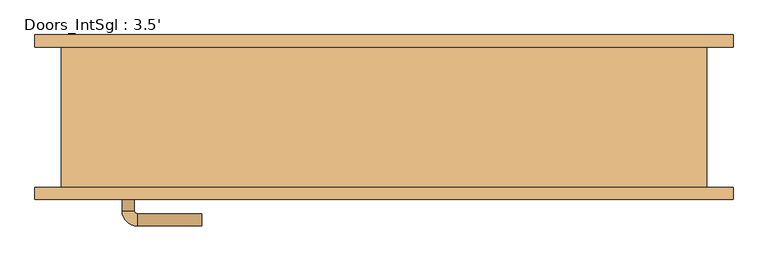
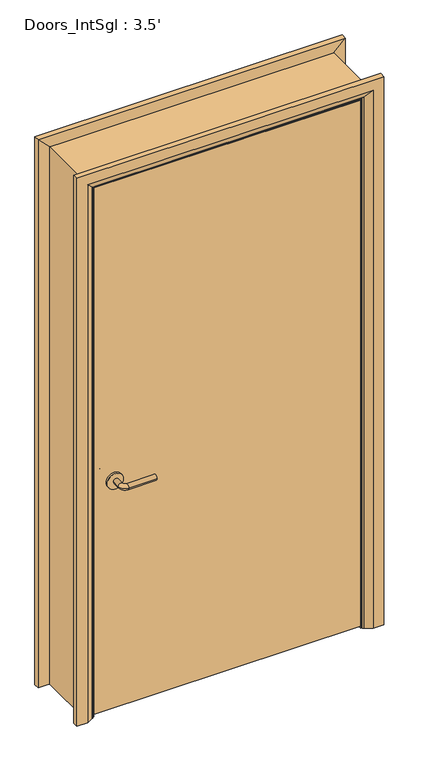
"""IFC4 building model written with IfcOpenShell, lengths in millimetres: door geometry, Doors_IntSgl : 3.5'."""

from ifc_helpers import new_model, si_unit, point, frame, frame_2d, origin, place, context, project, spatial, polyline, circle_curve, ellipse_curve, trimmed, segment, composite_curve, outline, extrude, faceted_brep, source, transform, mapped, element, save
from ifc_brep_helpers import plane_surface, cylinder_surface, revolved_surface, advanced_brep


def doors_intsgl_3_5_83ebdd9c(model_context):
    return source(origin(), model_context, "Body", "SolidModel", [
        advanced_brep(
        [(-426.4, -68.3, 900.0), (-406.4, -68.3, 900.0), (-426.4, -38.3, 900.0), (-406.4, -38.3, 900.0), (-401.4, -33.3, 900.0), (-401.4, -13.3, 900.0), (-296.4, -13.3, 900.0), (-296.4, -33.3, 900.0)],
        [
            (0, 1, circle_curve(frame((-416.4, -68.3, 900.0), z_axis=(0.0, -1.0, 0.0), x_axis=(1.0, 0.0, 0.0)), 10.0)),
            (1, 0, circle_curve(frame((-416.4, -68.3, 900.0), z_axis=(0.0, -1.0, 0.0), x_axis=(1.0, 0.0, 0.0)), 10.0)),
            (0, 2),
            (2, 3, circle_curve(frame((-416.4, -38.3, 900.0), z_axis=(0.0, -1.0, 0.0), x_axis=(1.0, 0.0, 0.0)), 10.0)),
            (3, 1),
            (3, 2, circle_curve(frame((-416.4, -38.3, 900.0), z_axis=(0.0, -1.0, 0.0), x_axis=(1.0, 0.0, 0.0)), 10.0)),
            (4, 3, circle_curve(frame((-401.4, -38.3, 900.0), z_axis=(0.0, 0.0, 1.0), x_axis=(-1.0, 0.0, 0.0)), 5.0)),
            (2, 5, circle_curve(frame((-401.4, -38.3, 900.0), z_axis=(0.0, 0.0, -1.0), x_axis=(-1.0, 0.0, 0.0)), 25.0)),
            (5, 4, circle_curve(frame((-401.4, -23.3, 900.0), z_axis=(-1.0, 0.0, 0.0), x_axis=(0.0, -1.0, 0.0)), 10.0)),
            (4, 5, circle_curve(frame((-401.4, -23.3, 900.0), z_axis=(-1.0, 0.0, 0.0), x_axis=(0.0, -1.0, 0.0)), 10.0)),
            (6, 7, circle_curve(frame((-296.4, -23.3, 900.0), z_axis=(1.0, 0.0, 0.0), x_axis=(0.0, -1.0, 0.0)), 10.0)),
            (7, 6, circle_curve(frame((-296.4, -23.3, 900.0), z_axis=(1.0, 0.0, 0.0), x_axis=(0.0, -1.0, 0.0)), 10.0)),
            (5, 6),
            (7, 4),
        ],
        [
            plane_surface(frame((-416.4, -68.3, 900.0), z_axis=(0.0, -1.0, 0.0), x_axis=(0.0, 0.0, 1.0))),
            cylinder_surface(frame((-416.4, -68.3, 900.0), z_axis=(0.0, -1.0, 0.0), x_axis=(1.0, 0.0, 0.0)), 10.0),
            revolved_surface(trimmed(ellipse_curve(frame((-416.4, -38.3, 900.0), z_axis=(0.0, -1.0, 0.0), x_axis=(1.0, 0.0, 0.0)), 10.0, 10.0), [point((-426.4, -38.3, 900.0))], [point((-406.4, -38.3, 900.0))], True, "CARTESIAN"), (-401.4, -38.3, 900.0), (0.0, 0.0, -1.0)),
            revolved_surface(trimmed(ellipse_curve(frame((-416.4, -38.3, 900.0), z_axis=(0.0, -1.0, 0.0), x_axis=(1.0, 0.0, 0.0)), 10.0, 10.0), [point((-406.4, -38.3, 900.0))], [point((-426.4, -38.3, 900.0))], True, "CARTESIAN"), (-401.4, -38.3, 900.0), (0.0, 0.0, -1.0)),
            plane_surface(frame((-296.4, -23.3, 900.0), z_axis=(1.0, 0.0, 0.0), x_axis=(0.0, 0.0, 1.0))),
            cylinder_surface(frame((-401.4, -23.3, 900.0), z_axis=(-1.0, 0.0, 0.0), x_axis=(0.0, -1.0, 0.0)), 10.0),
        ],
        [
            (0, [[1, 2]]),
            (1, [[-1, 3, 4, 5]]),
            (1, [[-2, -5, 6, -3]]),
            (2, [[7, -4, 8, 9]]),
            (3, [[-8, -6, -7, 10]]),
            (4, [[11, 12]]),
            (5, [[-9, 13, -12, 14]]),
            (5, [[-10, -14, -11, -13]]),
        ],
    ),
        extrude(outline(composite_curve([segment(trimmed(circle_curve(frame_2d((900.0, -418.9)), 30.0), [point((900.0, -448.9))], [point((900.0, -388.9))], False, "CARTESIAN"), True, "CONTINUOUS"), segment(trimmed(circle_curve(frame_2d((900.0, -418.9)), 30.0), [point((900.0, -388.9))], [point((900.0, -448.9))], False, "CARTESIAN"), True, "CONTINUOUS")], self_intersect=False)), frame((0.0, -76.3, 0.0), z_axis=(0.0, 1.0, 0.0), x_axis=(0.0, 0.0, 1.0)), (0.0, 0.0, 1.0), 8.0),
        advanced_brep(
        [(-426.4, -122.3, 900.0), (-406.4, -122.3, 900.0), (-406.4, -152.3, 900.0), (-426.4, -152.3, 900.0), (-401.4, -157.3, 900.0), (-401.4, -177.3, 900.0), (-296.4, -177.3, 900.0), (-296.4, -157.3, 900.0)],
        [
            (0, 1, circle_curve(frame((-416.4, -122.3, 900.0), z_axis=(0.0, 1.0, 0.0), x_axis=(1.0, 0.0, 0.0)), 10.0)),
            (1, 0, circle_curve(frame((-416.4, -122.3, 900.0), z_axis=(0.0, 1.0, 0.0), x_axis=(1.0, 0.0, 0.0)), 10.0)),
            (1, 2),
            (2, 3, circle_curve(frame((-416.4, -152.3, 900.0), z_axis=(0.0, 1.0, 0.0), x_axis=(1.0, 0.0, 0.0)), 10.0)),
            (3, 0),
            (3, 2, circle_curve(frame((-416.4, -152.3, 900.0), z_axis=(0.0, 1.0, 0.0), x_axis=(1.0, 0.0, 0.0)), 10.0)),
            (4, 5, circle_curve(frame((-401.4, -167.3, 900.0), z_axis=(-1.0, 0.0, 0.0), x_axis=(0.0, 1.0, 0.0)), 10.0)),
            (5, 3, circle_curve(frame((-401.4, -152.3, 900.0), z_axis=(0.0, 0.0, -1.0), x_axis=(-1.0, 0.0, 0.0)), 25.0)),
            (2, 4, circle_curve(frame((-401.4, -152.3, 900.0), z_axis=(0.0, 0.0, 1.0), x_axis=(-1.0, 0.0, 0.0)), 5.0)),
            (5, 4, circle_curve(frame((-401.4, -167.3, 900.0), z_axis=(-1.0, 0.0, 0.0), x_axis=(0.0, 1.0, 0.0)), 10.0)),
            (6, 7, circle_curve(frame((-296.4, -167.3, 900.0), z_axis=(1.0, 0.0, 0.0), x_axis=(0.0, 1.0, 0.0)), 10.0)),
            (7, 6, circle_curve(frame((-296.4, -167.3, 900.0), z_axis=(1.0, 0.0, 0.0), x_axis=(0.0, 1.0, 0.0)), 10.0)),
            (4, 7),
            (6, 5),
        ],
        [
            plane_surface(frame((-416.4, -122.3, 900.0), z_axis=(0.0, 1.0, 0.0), x_axis=(0.0, 0.0, 1.0))),
            cylinder_surface(frame((-416.4, -122.3, 900.0), z_axis=(0.0, 1.0, 0.0), x_axis=(1.0, 0.0, 0.0)), 10.0),
            revolved_surface(trimmed(ellipse_curve(frame((-416.4, -152.3, 900.0), z_axis=(0.0, -1.0, 0.0), x_axis=(1.0, 0.0, 0.0)), 10.0, 10.0), [point((-426.4, -152.3, 900.0))], [point((-406.4, -152.3, 900.0))], True, "CARTESIAN"), (-401.4, -152.3, 900.0), (0.0, 0.0, -1.0)),
            revolved_surface(trimmed(ellipse_curve(frame((-416.4, -152.3, 900.0), z_axis=(0.0, -1.0, 0.0), x_axis=(1.0, 0.0, 0.0)), 10.0, 10.0), [point((-406.4, -152.3, 900.0))], [point((-426.4, -152.3, 900.0))], True, "CARTESIAN"), (-401.4, -152.3, 900.0), (0.0, 0.0, -1.0)),
            plane_surface(frame((-296.4, -167.3, 900.0), z_axis=(1.0, 0.0, 0.0), x_axis=(0.0, 0.0, 1.0))),
            cylinder_surface(frame((-401.4, -167.3, 900.0), z_axis=(-1.0, 0.0, 0.0), x_axis=(0.0, 1.0, 0.0)), 10.0),
        ],
        [
            (0, [[1, 2]]),
            (1, [[3, 4, 5, -2]]),
            (1, [[-5, 6, -3, -1]]),
            (2, [[7, 8, -4, 9]]),
            (3, [[10, -9, -6, -8]]),
            (4, [[11, 12]]),
            (5, [[13, -11, 14, -7]]),
            (5, [[-14, -12, -13, -10]]),
        ],
    ),
        extrude(outline(composite_curve([segment(trimmed(circle_curve(frame_2d((900.0, -418.9)), 30.0), [point((900.0, -448.9))], [point((900.0, -388.9))], False, "CARTESIAN"), True, "CONTINUOUS"), segment(trimmed(circle_curve(frame_2d((900.0, -418.9)), 30.0), [point((900.0, -388.9))], [point((900.0, -448.9))], False, "CARTESIAN"), True, "CONTINUOUS")], self_intersect=False)), frame((0.0, -122.3, 0.0), z_axis=(0.0, 1.0, 0.0), x_axis=(0.0, 0.0, 1.0)), (0.0, 0.0, 1.0), 8.0),
        extrude(outline(polyline([(491.4, -76.3), (491.4, -114.3), (-491.4, -114.3), (-491.4, -76.3), (491.4, -76.3)])), frame((0.0, 0.0, 8.0), z_axis=(0.0, 0.0, 1.0), x_axis=(1.0, 0.0, 0.0)), (0.0, 0.0, 1.0), 2060.0),
        advanced_brep(
        [(568.4, -134.3, 0.0), (528.4, -134.3, 0.0), (502.4, -120.3, 0.0), (498.4, -114.3, 0.0), (568.4, -114.3, 0.0), (568.4, -114.3, 2145.0), (568.4, -134.3, 2145.0), (498.4, -114.3, 2075.0), (-498.4, -114.3, 2075.0), (-498.4, -114.3, 0.0), (-568.4, -114.3, 0.0), (-568.4, -114.3, 2145.0), (502.4, -120.3, 2079.0), (528.4, -134.3, 2105.0), (-568.4, -134.3, 2145.0), (-568.4, -134.3, 0.0), (-528.4, -134.3, 0.0), (-528.4, -134.3, 2105.0), (-502.4, -120.3, 0.0), (-502.4, -120.3, 2079.0)],
        [
            (0, 1),
            (1, 2),
            (2, 3, circle_curve(frame((506.4, -113.3, 0.0), z_axis=(0.0, 0.0, -1.0), x_axis=(1.0, 0.0, 0.0)), 8.0622577)),
            (3, 4),
            (4, 0),
            (4, 5),
            (5, 6),
            (6, 0),
            (3, 7),
            (7, 8),
            (8, 9),
            (9, 10),
            (10, 11),
            (11, 5),
            (2, 12),
            (12, 7, ellipse_curve(frame((506.4, -113.3, 2083.0), z_axis=(0.7071067811865475, 0.0, -0.7071067811865475), x_axis=(-0.7071067811865474, 0.0, -0.7071067811865476)), 11.4017543, 8.0622577)),
            (1, 13),
            (13, 12),
            (6, 14),
            (14, 15),
            (15, 16),
            (16, 17),
            (17, 13),
            (10, 15),
            (14, 11),
            (9, 18, circle_curve(frame((-506.4, -113.3, 0.0), z_axis=(0.0, 0.0, -1.0), x_axis=(-1.0, 0.0, 0.0)), 8.0622577)),
            (18, 16),
            (19, 18),
            (8, 19, ellipse_curve(frame((-506.4, -113.3, 2083.0), z_axis=(-0.7071067811865475, 0.0, -0.7071067811865475), x_axis=(-0.7071067811865474, 0.0, 0.7071067811865476)), 11.4017543, 8.0622577)),
            (19, 17),
            (12, 19),
        ],
        [
            plane_surface(frame((498.4, -114.3, 0.0), z_axis=(0.0, 0.0, -1.0), x_axis=(0.0, 1.0, 0.0))),
            plane_surface(frame((568.4, -134.3, 0.0), z_axis=(1.0, 0.0, 0.0), x_axis=(0.0, 0.0, 1.0))),
            plane_surface(frame((568.4, -114.3, 0.0), z_axis=(0.0, 1.0, 0.0), x_axis=(0.0, 0.0, 1.0))),
            cylinder_surface(frame((506.4, -113.3, 0.0), z_axis=(0.0, 0.0, -1.0), x_axis=(1.0, 0.0, 0.0)), 8.0622577),
            plane_surface(frame((502.4, -120.3, 0.0), z_axis=(-0.4740998230350126, -0.880471099922178, 0.0), x_axis=(0.0, 0.0, 1.0))),
            plane_surface(frame((528.4, -134.3, 0.0), z_axis=(0.0, -1.0, 0.0), x_axis=(0.0, 0.0, 1.0))),
            plane_surface(frame((-568.4, -134.3, 2145.0), z_axis=(-1.0, 0.0, 0.0), x_axis=(0.0, 0.0, -1.0))),
            plane_surface(frame((-498.4, -114.3, 0.0), z_axis=(0.0, 0.0, -1.0), x_axis=(0.0, 1.0, 0.0))),
            cylinder_surface(frame((-506.4, -113.3, 2075.0), z_axis=(0.0, 0.0, 1.0), x_axis=(-1.0, 0.0, 0.0)), 8.0622577),
            plane_surface(frame((-502.4, -120.3, 2079.0), z_axis=(0.47409982303501824, -0.8804710999221749, 0.0), x_axis=(0.0, 0.0, -1.0))),
            plane_surface(frame((568.4, -134.3, 2145.0), z_axis=(0.0, 0.0, 1.0), x_axis=(-1.0, 0.0, 0.0))),
            cylinder_surface(frame((498.4, -113.3, 2083.0), z_axis=(1.0, 0.0, 0.0), x_axis=(0.0, 0.0, 1.0)), 8.0622577),
            plane_surface(frame((502.4, -120.3, 2079.0), z_axis=(0.0, -0.8804710999221764, -0.4740998230350154), x_axis=(-1.0, 0.0, 0.0))),
        ],
        [
            (0, [[1, 2, 3, 4, 5]]),
            (1, [[6, 7, 8, -5]]),
            (2, [[9, 10, 11, 12, 13, 14, -6, -4]]),
            (3, [[15, 16, -9, -3]]),
            (4, [[17, 18, -15, -2]]),
            (5, [[-8, 19, 20, 21, 22, 23, -17, -1]]),
            (6, [[-13, 24, -20, 25]]),
            (7, [[-24, -12, 26, 27, -21]]),
            (8, [[28, -26, -11, 29]]),
            (9, [[-22, -27, -28, 30]]),
            (10, [[-14, -25, -19, -7]]),
            (11, [[31, -29, -10, -16]]),
            (12, [[-23, -30, -31, -18]]),
        ],
    ),
        extrude(outline(polyline([(0.0, -474.4), (2051.0, -474.4), (2051.0, 474.4), (0.0, 474.4), (0.0, 493.4), (2070.0, 493.4), (2070.0, -493.4), (0.0, -493.4), (0.0, -474.4)])), frame((0.0, -74.3, 0.0), z_axis=(0.0, 1.0, 0.0), x_axis=(0.0, 0.0, 1.0)), (0.0, 0.0, 1.0), 32.0),
        advanced_brep(
        [(-568.4, 134.3, 0.0), (-528.4, 134.3, 0.0), (-502.4, 120.3, 0.0), (-498.4, 114.3, 0.0), (-568.4, 114.3, 0.0), (-568.4, 114.3, 2145.0), (-568.4, 134.3, 2145.0), (-498.4, 114.3, 2075.0), (-502.4, 120.3, 2079.0), (-528.4, 134.3, 2105.0), (568.4, 134.3, 0.0), (568.4, 114.3, 0.0), (498.4, 114.3, 0.0), (502.4, 120.3, 0.0), (528.4, 134.3, 0.0), (568.4, 134.3, 2145.0), (528.4, 134.3, 2105.0), (502.4, 120.3, 2079.0), (498.4, 114.3, 2075.0), (568.4, 114.3, 2145.0)],
        [
            (0, 1),
            (1, 2),
            (2, 3, circle_curve(frame((-506.4, 113.3, 0.0), z_axis=(0.0, 0.0, -1.0), x_axis=(-1.0, 0.0, 0.0)), 8.0622577)),
            (3, 4),
            (4, 0),
            (4, 5),
            (5, 6),
            (6, 0),
            (3, 7),
            (7, 5),
            (2, 8),
            (8, 7, ellipse_curve(frame((-506.4, 113.3, 2083.0), z_axis=(-0.7071067811865475, 0.0, -0.7071067811865475), x_axis=(0.7071067811865474, 0.0, -0.7071067811865476)), 11.4017543, 8.0622577)),
            (1, 9),
            (9, 8),
            (6, 9),
            (10, 11),
            (11, 12),
            (12, 13, circle_curve(frame((506.4, 113.3, 0.0), z_axis=(0.0, 0.0, -1.0), x_axis=(1.0, 0.0, 0.0)), 8.0622577)),
            (13, 14),
            (14, 10),
            (15, 10),
            (14, 16),
            (16, 15),
            (13, 17),
            (17, 16),
            (12, 18),
            (18, 17, ellipse_curve(frame((506.4, 113.3, 2083.0), z_axis=(0.7071067811865475, 0.0, -0.7071067811865475), x_axis=(0.7071067811865474, 0.0, 0.7071067811865476)), 11.4017543, 8.0622577)),
            (11, 19),
            (19, 18),
            (15, 19),
            (5, 19),
            (15, 6),
            (7, 18),
            (8, 17),
            (9, 16),
        ],
        [
            plane_surface(frame((-498.4, 187.1010989, 0.0), z_axis=(0.0, 0.0, -1.0), x_axis=(1.0, 0.0, 0.0))),
            plane_surface(frame((-568.4, 134.3, 0.0), z_axis=(-1.0, 0.0, 0.0), x_axis=(0.0, 0.0, 1.0))),
            plane_surface(frame((-568.4, 114.3, 0.0), z_axis=(0.0, -1.0, 0.0), x_axis=(0.0, 0.0, 1.0))),
            cylinder_surface(frame((-506.4, 113.3, 0.0), z_axis=(0.0, 0.0, -1.0), x_axis=(-1.0, 0.0, 0.0)), 8.0622577),
            plane_surface(frame((-502.4, 120.3, 0.0), z_axis=(0.4740998230350183, 0.8804710999221749, 0.0), x_axis=(0.0, 0.0, 1.0))),
            plane_surface(frame((-528.4, 134.3, 0.0), z_axis=(0.0, 1.0, 0.0), x_axis=(0.0, 0.0, 1.0))),
            plane_surface(frame((498.4, 187.1010989, 0.0), z_axis=(0.0, 0.0, -1.0), x_axis=(-1.0, 0.0, 0.0))),
            plane_surface(frame((528.4, 134.3, 2105.0), z_axis=(0.0, 1.0, 0.0), x_axis=(0.0, 0.0, -1.0))),
            plane_surface(frame((502.4, 120.3, 2079.0), z_axis=(-0.4740998230350183, 0.8804710999221749, 0.0), x_axis=(0.0, 0.0, -1.0))),
            cylinder_surface(frame((506.4, 113.3, 2075.0), z_axis=(0.0, 0.0, 1.0), x_axis=(1.0, 0.0, 0.0)), 8.0622577),
            plane_surface(frame((568.4, 114.3, 2145.0), z_axis=(0.0, -1.0, 0.0), x_axis=(0.0, 0.0, -1.0))),
            plane_surface(frame((568.4, 134.3, 2145.0), z_axis=(1.0, 0.0, 0.0), x_axis=(0.0, 0.0, -1.0))),
            plane_surface(frame((-568.4, 134.3, 2145.0), z_axis=(0.0, 0.0, 1.0), x_axis=(1.0, 0.0, 0.0))),
            plane_surface(frame((-568.4, 114.3, 2145.0), z_axis=(0.0, -1.0, 0.0), x_axis=(1.0, 0.0, 0.0))),
            cylinder_surface(frame((-498.4, 113.3, 2083.0), z_axis=(-1.0, 0.0, 0.0), x_axis=(0.0, 0.0, 1.0)), 8.0622577),
            plane_surface(frame((-502.4, 120.3, 2079.0), z_axis=(0.0, 0.8804710999221749, -0.4740998230350183), x_axis=(1.0, 0.0, 0.0))),
            plane_surface(frame((-528.4, 134.3, 2105.0), z_axis=(0.0, 1.0, 0.0), x_axis=(1.0, 0.0, 0.0))),
        ],
        [
            (0, [[1, 2, 3, 4, 5]]),
            (1, [[6, 7, 8, -5]]),
            (2, [[9, 10, -6, -4]]),
            (3, [[11, 12, -9, -3]]),
            (4, [[13, 14, -11, -2]]),
            (5, [[-8, 15, -13, -1]]),
            (6, [[16, 17, 18, 19, 20]]),
            (7, [[21, -20, 22, 23]]),
            (8, [[-22, -19, 24, 25]]),
            (9, [[-24, -18, 26, 27]]),
            (10, [[-26, -17, 28, 29]]),
            (11, [[-28, -16, -21, 30]]),
            (12, [[31, -30, 32, -7]]),
            (13, [[33, -29, -31, -10]]),
            (14, [[34, -27, -33, -12]]),
            (15, [[35, -25, -34, -14]]),
            (16, [[-32, -23, -35, -15]]),
        ],
    ),
        faceted_brep([(-493.4, -114.3, 0.0), (-525.4, -114.3, 0.0), (-525.4, 114.3, 0.0), (-493.4, 114.3, 0.0), (-493.4, 114.3, 2070.0), (-493.4, -114.3, 2070.0), (-525.4, 114.3, 2102.0), (-525.4, -114.3, 2102.0), (493.4, -114.3, 0.0), (493.4, 114.3, 0.0), (525.4, 114.3, 0.0), (525.4, -114.3, 0.0), (493.4, -114.3, 2070.0), (525.4, -114.3, 2102.0), (525.4, 114.3, 2102.0), (493.4, 114.3, 2070.0)], [[[0, 1, 2, 3]], [[3, 4, 5, 0]], [[2, 6, 4, 3]], [[1, 7, 6, 2]], [[0, 5, 7, 1]], [[8, 9, 10, 11]], [[12, 8, 11, 13]], [[13, 11, 10, 14]], [[14, 10, 9, 15]], [[15, 9, 8, 12]], [[4, 15, 12, 5]], [[6, 14, 15, 4]], [[7, 13, 14, 6]], [[5, 12, 13, 7]]]),
    ])


if __name__ == "__main__":
    model = new_model("IFC4")
    model_context = context("Model", 3, world=origin())
    ifc_project = project(units=[si_unit("LENGTHUNIT", "METRE", prefix="MILLI")], contexts=[model_context])
    site = spatial("IfcSite", under=ifc_project)
    building = spatial("IfcBuilding", under=site)
    placement = place(None, origin())
    doors_intsgl_3_5_shape = doors_intsgl_3_5_83ebdd9c(model_context)
    element("IfcDoor", 1, ObjectType="Doors_IntSgl : 3.5'", at=placement, inside=building, context=model_context, shape_type="MappedRepresentation", body=[
        mapped(doors_intsgl_3_5_shape, transform((0.0, 0.0, 0.0), x_axis=(1.0, 0.0, 0.0), y_axis=(0.0, 1.0, 0.0), z_axis=(0.0, 0.0, 1.0))),
    ])
    save(model, "model.ifc")

# Revit data of these elements
# Type "Doors_IntSgl : 3.5'"
#   Type Mark = "51"
#   Type Comments = "Internal Single"
#   Operation = "SingleSwingRight"
#   Manufacturer = "Revit"
#   Keynote = "L20"
#   Description = "Internal Single Door"
#   Analytic Construction = "Metal"
#   UnderCut = 0.026247 ft
#   Tolerance = 0.006562 ft
#   Thickness = 0.124672 ft
#   Thermal Resistance (R) = 0.270117 (m²·K)/W
#   Structural Tolerance = 0.026247 ft
#   StopDepth = 0.104987 ft
#   Stop Thickness = 0.062336 ft
#   Rough Width = 3.5 ft
#   Rough Height = 6.922572 ft
#   Height to Top Lock Rail = 3.28084 ft
#   Heat Transfer Coefficient (U) = 3.7021 W/(m²·K)
#   Handle Z Distance = 2.952756 ft
#   Handle X Distance = 0.246063 ft
#   Frame Thickness = 0.104987 ft
#   Door Panel Width = 3.224409 ft
#   Door Panel Thickness = 0.124672 ft
#   Door Panel Offset = 0.0 ft
#   Height = 6.922572 ft
#   Width = 3.5 ft
#   Door Panel Height = 6.75853 ft
#   Architrave Setback = 0.016404 ft
#   Vis - Ironmongery = yes
#   Material Ironmongery = Door - Handle
#   Material Frame = Door - Frame/Mullion (1)
#   Material Door = Door - Panel
#   Material Architrave = Door - Architrave
#   Visual Light Transmittance = 0
#   Solar Heat Gain Coefficient = 0
#   Function = (empty or 0)
#   Wall Closure = (empty or 0)
# Element 1 (IfcDoor, "Doors_IntSgl : 3.5'")
#   Materials on its faces: "Door - Architrave", "Door - Handle", "Door - Frame/Mullion (1)", "Door - Panel"
# Materials
#   "Door - Handle": colour RGB 0 0 0, transparency 0, Keynote = "P21", Cost = 0
#   "Door - Frame/Mullion (1)": class "Wood", colour RGB 212 179 113, transparency 0, Keynote = "L20", Cost = 0
#   "Door - Panel": class "Wood", colour RGB 210 159 95, transparency 0, Keynote = "L20", Cost = 0
#   "Door - Architrave": class "Wood", colour RGB 154 90 5, transparency 0, Keynote = "P20", Cost = 0
